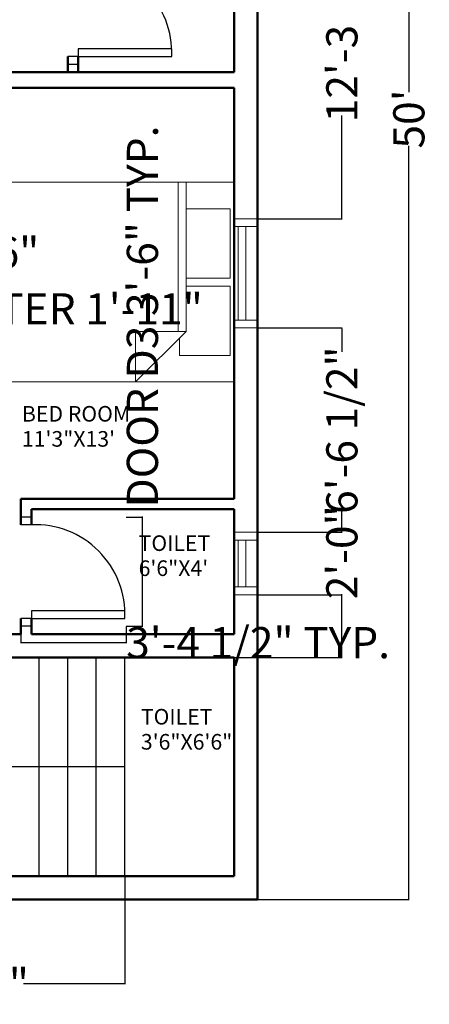
# Model space of a CAD drawing. Units: inches. Extents: x -51 to 1118, y -44 to 791.
# Tile 3 of 8: x 249 to 406, y -34 to 344. Entities that reach past the tile are written whole.
import ezdxf

# ---------------------------------------------------------------- set-up
doc = ezdxf.new("R2010")
doc.units = ezdxf.units.IN
doc.header["$MEASUREMENT"] = 0
for name, color, linetype, lineweight in [('A-ANNO-DIMS', 2, 'Continuous', 18), ('A-AREA-IDEN', 7, 'Continuous', 18), ('A-DOOR', 3, 'Continuous', 25), ('A-FLOR-STRS', 7, 'Continuous', 25), ('A-FURN', 8, 'Continuous', 18), ('A-GLAZ', 4, 'Continuous', 18), ('A-WALL', 7, 'Continuous', 50)]:
    doc.layers.add(name, color=color, linetype=linetype, lineweight=lineweight)
doc.styles.get("Standard").update_dxf_attribs({"font": 'arial.ttf'})
doc.dimstyles.get("Standard").update_dxf_attribs({"dimtxt": 12, "dimasz": 0.18, "dimexe": 0.18, "dimexo": 0.0625, "dimgap": 0.09, "dimtad": 0, "dimdec": 1, "dimzin": 0, "dimdsep": 46, "dimlunit": 3, "dimtxsty": 'Standard', "dimcen": 0.09, "dimadec": 0, "dimazin": 0, "dimtfac": 1, "dimtdec": 1, "dimtofl": 0, "dimtmove": 0, "dimatfit": 3, "dimfxl": 1, "dimtolj": 1, "dimtzin": 0, "dimarcsym": 0})

# ---------------------------------------------------------------- blocks, each defined once
blk = doc.blocks.new('Bed - Queen')
for p, q in [((0, -80.00003), (0, 0)), ((0, 0), (59.99999, 0)), ((59.99999, 0), (59.99999, -80.00003)), ((7.99999, -1.2), (28.79998, -1.2)), ((7.99999, -14.4), (7.99999, -1.2)), ((28.79998, -1.2), (28.79998, -14.4)), ((31.19999, -1.2), (51.99999, -1.2)), ((31.19999, -14.4), (31.19999, -1.2)), ((51.99999, -1.2), (51.99999, -16.4)), ((0, -14.4), (44.8, -14.4)), ((59.99999, -29.6), (44.8, -14.4)), ((44.8, -14.4), (44.8, -29.6)), ((44.8, -16.8), (0, -16.8)), ((51.99999, -16.4), (46.79936, -16.4)), ((44.8, -29.6), (59.99999, -29.6)), ((59.99999, -80.00003), (0, -80.00003))]:
    blk.add_line(p, q)
blk = doc.blocks.new('*D9')
at = {"layer": 'A-ANNO-DIMS', "color": 0, "lineweight": -2, "transparency": 16777216}
for p, q in [((340.08, 605.94), (398.42, 605.94)), ((398.24, 605.76), (398.24, 316.21)), ((398.24, 6.12), (398.24, 295.67)), ((340.08, 5.94), (398.42, 5.94))]:
    blk.add_line(p, q, dxfattribs=at)
at = {"layer": 'A-ANNO-DIMS', "color": 0, "transparency": 16777216}
for points in [[(398.21, 605.76), (398.27, 605.76), (398.24, 605.94)], [(398.21, 6.12), (398.27, 6.12), (398.24, 5.94)]]:
    blk.add_solid(points, dxfattribs=at)
at = {"layer": 'Defpoints', "color": 0, "transparency": 16777216}
for p in [(340.02, 605.94), (340.02, 5.94), (398.24, 5.94)]:
    blk.add_point(p, dxfattribs=at)
at = {"layer": 'A-ANNO-DIMS', "color": 0, "transparency": 16777216, "insert": (398.24, 305.94), "char_height": 12, "attachment_point": 5, "rotation": 90}
blk.add_mtext("\\A1;50'", dxfattribs=at)
blk = doc.blocks.new('WIN-36IN')
for p, q in [((9, 42), (0, 42)), ((9, 39), (0, 39)), ((0, 39), (0, 3)), ((4.5, 3), (4.5, 39)), ((7.5, 3), (7.5, 39)), ((9, 3), (9, 39)), ((0, 3), (9, 3)), ((0, 0), (9, 0))]:
    blk.add_line(p, q)
blk = doc.blocks.new('WIN-18IN')
for p, q in [((9, 24), (0, 24)), ((0, 21), (0, 3)), ((9, 21), (0, 21)), ((1.5, 21), (1.5, 3)), ((4.5, 21), (4.5, 3)), ((9, 3), (9, 21)), ((0, 3), (9, 3)), ((0, 0), (9, 0))]:
    blk.add_line(p, q)
blk = doc.blocks.new('DOOR-36IN-FRAME-4IN')
for p, q in [((4, 42), (0, 42)), ((4, 39), (0, 39)), ((4, 3), (0, 3)), ((4, 0), (0, 0))]:
    blk.add_line(p, q)
blk.add_lwpolyline([(4, 3), (40, 3), (40, 6), (4, 6)], close=True)
blk.add_arc((5.5, 4.5), 34.53, 357.5104, 92.4896)
blk = doc.blocks.new('*D24')
at = {"layer": 'A-ANNO-DIMS', "color": 0, "lineweight": -2, "transparency": 16777216}
for p, q in [((289.5, 152.94), (295.92, 152.94)), ((295.74, 152.94), (295.74, 153.12)), ((295.74, 111.12), (295.74, 152.76)), ((289.5, 110.94), (295.92, 110.94))]:
    blk.add_line(p, q, dxfattribs=at)
at = {"layer": 'A-ANNO-DIMS', "color": 0, "transparency": 16777216}
for points in [[(295.71, 152.76), (295.77, 152.76), (295.74, 152.94)], [(295.71, 111.12), (295.77, 111.12), (295.74, 110.94)]]:
    blk.add_solid(points, dxfattribs=at)
at = {"layer": 'Defpoints', "color": 0, "transparency": 16777216}
for p in [(289.44, 152.94), (295.74, 152.94), (289.44, 110.94)]:
    blk.add_point(p, dxfattribs=at)
at = {"layer": 'A-ANNO-DIMS', "color": 0, "transparency": 16777216, "insert": (295.74, 230), "char_height": 12, "attachment_point": 5, "rotation": 90}
blk.add_mtext('\\A1;DOOR D3 3\'-6" TYP.', dxfattribs=at)
blk = doc.blocks.new('*D25')
at = {"layer": 'A-ANNO-DIMS', "color": 0, "lineweight": -2, "transparency": 16777216}
for p, q in [((249.02, 110.88), (249.02, 104.46)), ((289.44, 110.88), (289.44, 104.46)), ((249.2, 104.64), (289.26, 104.64)), ((289.44, 104.64), (289.62, 104.64))]:
    blk.add_line(p, q, dxfattribs=at)
at = {"layer": 'A-ANNO-DIMS', "color": 0, "transparency": 16777216}
for points in [[(249.2, 104.67), (249.2, 104.61), (249.02, 104.64)], [(289.26, 104.67), (289.26, 104.61), (289.44, 104.64)]]:
    blk.add_solid(points, dxfattribs=at)
at = {"layer": 'Defpoints', "color": 0, "transparency": 16777216}
for p in [(249.02, 110.94), (289.44, 110.94), (289.44, 104.64)]:
    blk.add_point(p, dxfattribs=at)
at = {"layer": 'A-ANNO-DIMS', "color": 0, "transparency": 16777216, "insert": (340.26, 104.64), "char_height": 12, "attachment_point": 5}
blk.add_mtext('\\A1;3\'-4 1/2" TYP.', dxfattribs=at)
blk = doc.blocks.new('*D30')
at = {"layer": 'A-ANNO-DIMS', "color": 0, "lineweight": -2, "transparency": 16777216}
for p, q in [((156.48, 229.58), (156.48, 233.14)), ((156.66, 232.96), (179.3, 232.96)), ((179.48, 229.58), (179.48, 233.14)), ((179.48, 232.96), (179.66, 232.96))]:
    blk.add_line(p, q, dxfattribs=at)
at = {"layer": 'A-ANNO-DIMS', "color": 0, "transparency": 16777216}
for points in [[(156.66, 232.99), (156.66, 232.93), (156.48, 232.96)], [(179.3, 232.99), (179.3, 232.93), (179.48, 232.96)]]:
    blk.add_solid(points, dxfattribs=at)
at = {"layer": 'Defpoints', "color": 0, "transparency": 16777216}
for p in [(179.48, 232.96), (156.48, 229.51), (179.48, 229.51)]:
    blk.add_point(p, dxfattribs=at)
at = {"layer": 'A-ANNO-DIMS', "color": 0, "transparency": 16777216, "insert": (250.58, 232.96), "char_height": 12, "attachment_point": 5}
blk.add_mtext('\\A1;COMPUTER 1\'-11"', dxfattribs=at)
blk = doc.blocks.new('*D36')
at = {"layer": 'A-ANNO-DIMS', "color": 0, "lineweight": -2, "transparency": 16777216}
for p, q in [((79.8, 262.73), (79.8, 254.48)), ((134, 262.73), (134, 254.48)), ((79.98, 254.66), (133.82, 254.66)), ((134, 254.66), (134.18, 254.66))]:
    blk.add_line(p, q, dxfattribs=at)
at = {"layer": 'A-ANNO-DIMS', "color": 0, "transparency": 16777216}
for points in [[(79.98, 254.69), (79.98, 254.63), (79.8, 254.66)], [(133.82, 254.69), (133.82, 254.63), (134, 254.66)]]:
    blk.add_solid(points, dxfattribs=at)
at = {"layer": 'Defpoints', "color": 0, "transparency": 16777216}
for p in [(79.8, 262.79), (134, 262.79), (134, 254.66)]:
    blk.add_point(p, dxfattribs=at)
at = {"layer": 'A-ANNO-DIMS', "color": 0, "transparency": 16777216, "insert": (196.54, 254.66), "char_height": 12, "attachment_point": 5}
blk.add_mtext('\\A1;LOVESEAT 4\'-6"', dxfattribs=at)
blk = doc.blocks.new('*D50')
at = {"layer": 'A-ANNO-DIMS', "color": 0, "lineweight": -2, "transparency": 16777216}
for p, q in [((340.08, 123.08), (372.65, 123.08)), ((372.47, 123.08), (372.47, 123.26)), ((372.47, 99.12), (372.47, 122.9)), ((331.08, 98.94), (372.65, 98.94))]:
    blk.add_line(p, q, dxfattribs=at)
at = {"layer": 'A-ANNO-DIMS', "color": 0, "transparency": 16777216}
for points in [[(372.44, 122.9), (372.5, 122.9), (372.47, 123.08)], [(372.44, 99.12), (372.5, 99.12), (372.47, 98.94)]]:
    blk.add_solid(points, dxfattribs=at)
at = {"layer": 'Defpoints', "color": 0, "transparency": 16777216}
for p in [(340.02, 123.08), (372.47, 123.08), (331.02, 98.94)]:
    blk.add_point(p, dxfattribs=at)
at = {"layer": 'A-ANNO-DIMS', "color": 0, "transparency": 16777216, "insert": (372.47, 139.4), "char_height": 12, "attachment_point": 5, "rotation": 90}
blk.add_mtext('\\A1;2\'-0"', dxfattribs=at)
blk = doc.blocks.new('*D51')
at = {"layer": 'A-ANNO-DIMS', "color": 0, "lineweight": -2, "transparency": 16777216}
for p, q in [((340.08, 225.63), (372.65, 225.63)), ((372.47, 225.45), (372.47, 216.41)), ((372.47, 147.26), (372.47, 156.3)), ((340.08, 147.08), (372.65, 147.08))]:
    blk.add_line(p, q, dxfattribs=at)
at = {"layer": 'A-ANNO-DIMS', "color": 0, "transparency": 16777216}
for points in [[(372.44, 225.45), (372.5, 225.45), (372.47, 225.63)], [(372.44, 147.26), (372.5, 147.26), (372.47, 147.08)]]:
    blk.add_solid(points, dxfattribs=at)
at = {"layer": 'Defpoints', "color": 0, "transparency": 16777216}
for p in [(340.02, 225.63), (372.47, 225.63), (340.02, 147.08)]:
    blk.add_point(p, dxfattribs=at)
at = {"layer": 'A-ANNO-DIMS', "color": 0, "transparency": 16777216, "insert": (372.47, 186.35), "char_height": 12, "attachment_point": 5, "rotation": 90}
blk.add_mtext('\\A1;6\'-6 1/2"', dxfattribs=at)
blk = doc.blocks.new('*D52')
at = {"layer": 'A-ANNO-DIMS', "color": 0, "lineweight": -2, "transparency": 16777216}
for p, q in [((340.08, 415.22), (372.65, 415.22)), ((372.47, 415.04), (372.47, 375.54)), ((372.47, 267.81), (372.47, 307.31)), ((340.08, 267.63), (372.65, 267.63))]:
    blk.add_line(p, q, dxfattribs=at)
at = {"layer": 'A-ANNO-DIMS', "color": 0, "transparency": 16777216}
for points in [[(372.44, 415.04), (372.5, 415.04), (372.47, 415.22)], [(372.44, 267.81), (372.5, 267.81), (372.47, 267.63)]]:
    blk.add_solid(points, dxfattribs=at)
at = {"layer": 'Defpoints', "color": 0, "transparency": 16777216}
for p in [(340.02, 415.22), (372.47, 415.22), (340.02, 267.63)]:
    blk.add_point(p, dxfattribs=at)
at = {"layer": 'A-ANNO-DIMS', "color": 0, "transparency": 16777216, "insert": (372.47, 341.42), "char_height": 12, "attachment_point": 5, "rotation": 90}
blk.add_mtext('\\A1;12\'-3 1/2"', dxfattribs=at)
blk = doc.blocks.new('*D58')
at = {"layer": 'A-ANNO-DIMS', "color": 0, "lineweight": -2, "transparency": 16777216}
for p, q in [((179.02, 14.88), (179.02, -26.69)), ((289.02, 14.88), (289.02, -26.69)), ((179.2, -26.51), (217.98, -26.51)), ((288.84, -26.51), (250.06, -26.51))]:
    blk.add_line(p, q, dxfattribs=at)
at = {"layer": 'A-ANNO-DIMS', "color": 0, "transparency": 16777216}
for points in [[(179.2, -26.48), (179.2, -26.54), (179.02, -26.51)], [(288.84, -26.48), (288.84, -26.54), (289.02, -26.51)]]:
    blk.add_solid(points, dxfattribs=at)
at = {"layer": 'Defpoints', "color": 0, "transparency": 16777216}
for p in [(179.02, 14.94), (289.02, 14.94), (179.02, -26.51)]:
    blk.add_point(p, dxfattribs=at)
at = {"layer": 'A-ANNO-DIMS', "color": 0, "transparency": 16777216, "insert": (234.02, -26.51), "char_height": 12, "attachment_point": 5}
blk.add_mtext('\\A1;9\'-2"', dxfattribs=at)

msp = doc.modelspace()

# ---------------------------------------------------------------- linework, layer by layer
at = {"layer": 'A-FLOR-STRS'}
for p, q in [((256.02, 14.94), (256.02, 98.94)), ((267.02, 14.94), (267.02, 98.94)), ((278.02, 14.94), (278.02, 98.94)), ((289.02, 14.94), (289.02, 98.94)), ((289.02, 56.94), (179.02, 56.94))]:
    msp.add_line(p, q, dxfattribs=at)
at = {"layer": 'A-WALL'}
for p, q in [((331.02, 323.94), (331.02, 394.94)), ((267.02, 323.94), (267.02, 329.94)), ((271.02, 323.94), (271.02, 329.94)), ((331.02, 323.94), (235.02, 323.94)), ((331.02, 317.94), (235.02, 317.94)), ((331.02, 159.94), (331.02, 317.94)), ((331.02, 159.94), (249.02, 159.94)), ((249.02, 149.94), (249.02, 159.94)), ((331.02, 155.94), (253.02, 155.94)), ((253.02, 149.94), (253.02, 155.94)), ((331.02, 107.94), (331.02, 155.94)), ((249.02, 107.94), (249.02, 113.94)), ((253.02, 107.94), (253.02, 113.94)), ((249.02, 107.94), (193.02, 107.94)), ((331.02, 107.94), (253.02, 107.94)), ((331.02, 98.94), (79.02, 98.94)), ((331.02, 14.94), (331.02, 98.94)), ((37.02, 14.94), (331.02, 14.94))]:
    msp.add_line(p, q, dxfattribs=at)
msp.add_lwpolyline([(145.02, 605.94), (28.02, 605.94), (28.02, 5.94), (340.02, 5.94), (340.02, 605.94), (181.02, 605.94)], dxfattribs=at)

# ---------------------------------------------------------------- block references
at = {"layer": 'A-DOOR'}
for p in [(267.02, 326.94), (249.02, 110.94)]:
    msp.add_blockref('DOOR-36IN-FRAME-4IN', p, dxfattribs=at)
at = {"layer": 'A-FURN', "xscale": 1.279882060607878, "yscale": 1.279882060607878, "zscale": 1.279882060607878, "rotation": 270}
msp.add_blockref('Bed - Queen', (331.02, 281.65), dxfattribs=at)
at = {"layer": 'A-GLAZ', "rotation": 180}
msp.add_blockref('WIN-36IN', (340.02, 267.63), dxfattribs=at)
at = {"layer": 'A-GLAZ'}
msp.add_blockref('WIN-18IN', (331.02, 123.08), dxfattribs=at)

# ---------------------------------------------------------------- texts
at = {"layer": 'A-AREA-IDEN'}
for s, p in [('BED ROOM', (249.39, 189.62)), ('11\'3"X13\'', (249.39, 179.98)), ('TOILET', (294.29, 139.9)), ('6\'6"X4\'', (294.29, 130.27)), ('TOILET', (295.15, 73.17)), ('3\'6"X6\'6"', (295.15, 63.53))]:
    msp.add_text(s, height=6, dxfattribs=at).set_placement(p)

# ---------------------------------------------------------------- dimensions: what is measured, and where the dimension line sits
at = {"layer": 'A-ANNO-DIMS'}
for base, p1, p2, override, picture, middle in [((398.24, 5.94), (340.02, 605.94), (340.02, 5.94), {"dimclrd": 0, "dimclre": 0, "dimclrt": 0}, '*D9', (398.24, 305.94)), ((372.47, 415.22), (340.02, 267.63), (340.02, 415.22), {"dimdec": 1, "dimlfac": 1, "dimrnd": 0, "dimzin": 1, "dimdsep": 46, "dimlunit": 4, "dimfrac": 2}, '*D52', (372.47, 341.42)), ((372.4717, 225.6282), (340.0217, 147.0816), (340.0217, 225.6282), {"dimdec": 1, "dimlfac": 1, "dimrnd": 0, "dimzin": 1, "dimdsep": 46, "dimlunit": 4, "dimfrac": 2}, '*D51', (372.4717, 186.3549)), ((372.47, 123.08), (331.02, 98.94), (340.02, 123.08), {"dimdec": 1, "dimlfac": 1, "dimrnd": 0, "dimzin": 1, "dimdsep": 46, "dimlunit": 4, "dimfrac": 2}, '*D50', (372.47, 139.4))]:
    dim = msp.add_linear_dim(base=base, p1=p1, p2=p2, angle=90, dimstyle='Standard', override=override, dxfattribs=at)
    dim.commit()
    dim.dimension.update_dxf_attribs({"geometry": picture, "text_midpoint": middle})
dim = msp.add_linear_dim(base=(295.74, 152.94), p1=(289.44, 110.94), p2=(289.44, 152.94), angle=90, text='DOOR D3 <> TYP.', dimstyle='Standard', override={"dimdec": 1, "dimlfac": 1, "dimrnd": 0, "dimzin": 1, "dimdsep": 46, "dimlunit": 4, "dimfrac": 2}, dxfattribs=at)
dim.commit()
dim.dimension.update_dxf_attribs({"geometry": '*D24', "text_midpoint": (295.74, 230)})
for base, p1, p2, text, picture, middle in [((134, 254.66), (79.8, 262.79), (134, 262.79), 'LOVESEAT <>', '*D36', (196.54, 254.66)), ((179.48, 232.96), (156.48, 229.51), (179.48, 229.51), 'COMPUTER <>', '*D30', (250.58, 232.96)), ((289.44, 104.64), (249.02, 110.94), (289.44, 110.94), '<> TYP.', '*D25', (340.26, 104.64))]:
    dim = msp.add_linear_dim(base=base, p1=p1, p2=p2, text=text, dimstyle='Standard', override={"dimdec": 1, "dimlfac": 1, "dimrnd": 0, "dimzin": 1, "dimdsep": 46, "dimlunit": 4, "dimfrac": 2}, dxfattribs=at)
    dim.commit()
    dim.dimension.update_dxf_attribs({"geometry": picture, "text_midpoint": middle})
dim = msp.add_linear_dim(base=(179.02, -26.51), p1=(289.02, 14.94), p2=(179.02, 14.94), dimstyle='Standard', override={"dimdec": 1, "dimlfac": 1, "dimrnd": 0, "dimzin": 1, "dimdsep": 46, "dimlunit": 4, "dimfrac": 2}, dxfattribs=at)
dim.commit()
dim.dimension.update_dxf_attribs({"geometry": '*D58', "text_midpoint": (234.02, -26.51)})

doc.saveas('drawing.dxf')
